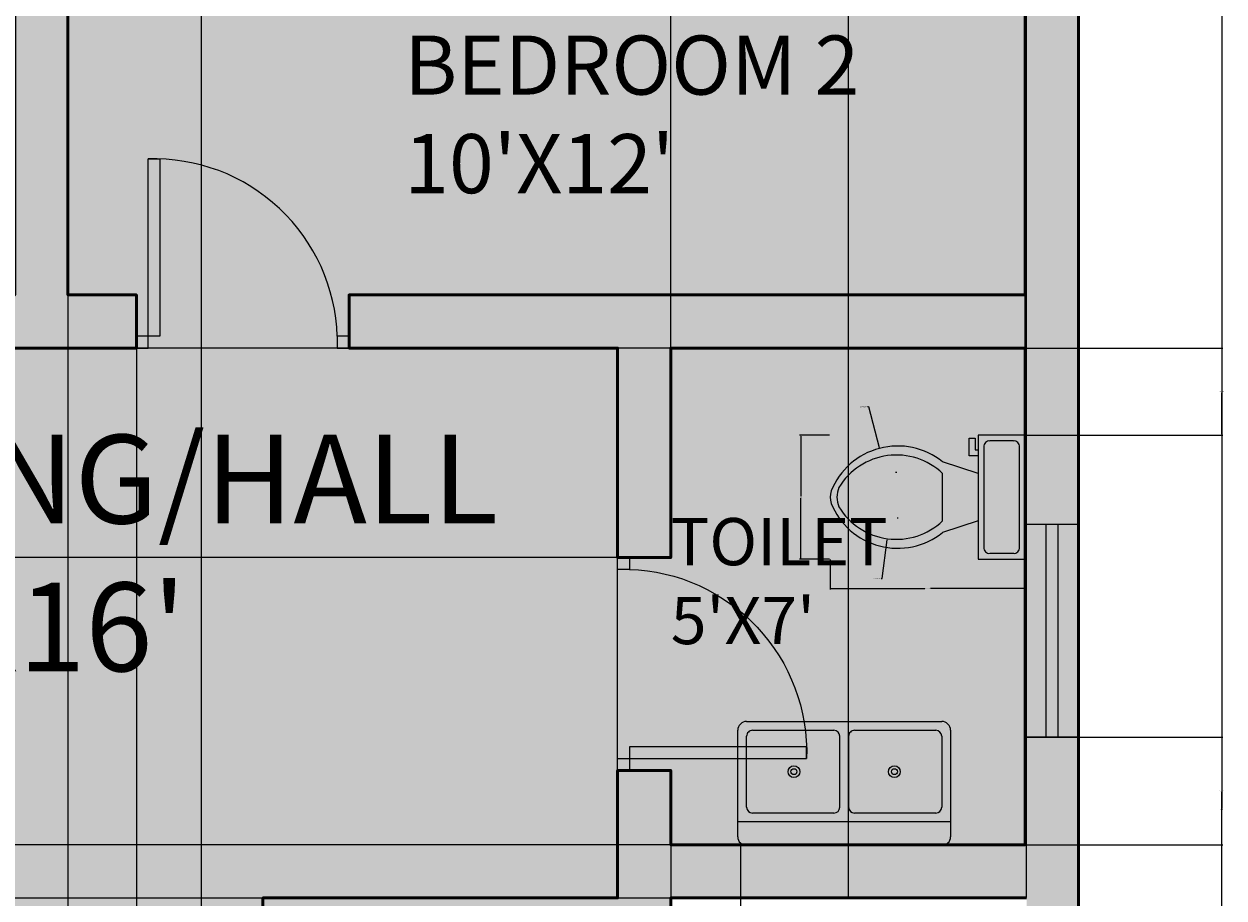
# Model space of a CAD drawing. Units: inches. Extents: x -494 to 1275, y 12 to 1194.
# Tile 3 of 8: x 293 to 496, y 596 to 743. Entities that reach past the tile are written whole.
import ezdxf

# ---------------------------------------------------------------- set-up
doc = ezdxf.new("R2010")
doc.units = ezdxf.units.IN
doc.header["$MEASUREMENT"] = 0
for name, color, linetype, lineweight in [('A-ANNO-DIMS', 2, 'Continuous', 18), ('A-AREA-IDEN', 7, 'Continuous', 25), ('A-DOOR', 3, 'Continuous', 25), ('A-DOOR-PATT', 7, 'Continuous', 13), ('A-FLOR-FIXT', 8, 'Continuous', 18), ('A-GLAZ', 4, 'Continuous', 18), ('A-GLAZ-FRAM-PATT', 7, 'Continuous', 13), ('A-GLAZ-GLAS-PATT', 4, 'Continuous', 13), ('A-WALL', 7, 'Continuous', 50)]:
    doc.layers.add(name, color=color, linetype=linetype, lineweight=lineweight)
doc.layers.add('A-FLOR-PATT', color=51, linetype='Continuous', lineweight=13, true_color=0xf8f6b0)
doc.layers.add('A-WALL-PATT', color=251, linetype='Continuous', lineweight=13, true_color=0x636466)
doc.styles.get("Standard").update_dxf_attribs({"font": 'arial.ttf'})
doc.dimstyles.get("Standard").update_dxf_attribs({"dimtxt": 0.18, "dimasz": 0.18, "dimexe": 0.18, "dimexo": 0.0625, "dimgap": 0.09, "dimtad": 0, "dimtih": 1, "dimtoh": 1, "dimdec": 4, "dimzin": 0, "dimdsep": 46, "dimlunit": 4, "dimtxsty": 'Standard', "dimcen": 0.09, "dimadec": 0, "dimazin": 0, "dimtfac": 1, "dimtdec": 4, "dimtofl": 0, "dimtmove": 0, "dimatfit": 3, "dimfxl": 1, "dimtolj": 1, "dimtzin": 0, "dimarcsym": 0})

# ---------------------------------------------------------------- blocks, each defined once
blk = doc.blocks.new('Toilet - top')
for p, q in [((9.5, -6), (9.5, -2)), ((-8, -8.5), (-8, -8)), ((-7, -8), (-7, -9.5)), ((-4, -8), (-6, -14)), ((4, -8), (6, -14)), ((-10, -8.5), (-8, -8.5)), ((-10, -9.5), (-10, -8.5)), ((-7, -9.5), (-10, -9.5)), ((4, -14), (-4, -14))]:
    blk.add_line(p, q)
blk.add_lwpolyline([(10.5, -8), (10.5, 0), (-10.5, 0), (-10.5, -8)], close=True)
for points in [[(-9.5, -2), (-9.5, -6)], [(8.5, -1), (-8.5, -1)], [(-8.5, -7), (8.5, -7)]]:
    blk.add_lwpolyline(points)
for centre, radius, start, end in [((-8.62, -1.88), 0.884, 81.8699, 188.1301), ((8.62, -1.88), 0.884, 351.8699, 98.1301), ((-8.62, -6.12), 0.884, 171.8699, 278.1301), ((8.62, -6.12), 0.884, 261.8699, 8.1301), ((3.52, -21.58), 12.17, 141.4691, 247.9714), ((4.2, -21.82), 11.33, 136.3677, 238.9468), ((-3.52, -21.58), 12.17, 292.0284, 38.5307), ((-4.2, -21.82), 11.33, 301.053, 43.6321), ((0, -27.88), 4, 245.7318, 294.2682), ((0, -29), 4, 254.8605, 285.1395)]:
    blk.add_arc(centre, radius, start, end)
blk = doc.blocks.new('Sink-double - 36 in top')
for p, q in [((-18, -4), (18, -4)), ((-0.75, -18.5), (-0.75, -6.5)), ((0.75, -6.5), (0.75, -18.5))]:
    blk.add_line(p, q)
for points in [[(-16.5, 0), (16.5, 0)], [(-18, -19.5), (-18, -1.5)], [(18, -1.5), (18, -19.5)], [(-15.5, -5.5), (-1.75, -5.5)], [(1.75, -5.5), (15.5, -5.5)], [(-16.5, -18.5), (-16.5, -6.5)], [(16.5, -6.5), (16.5, -18.5)], [(-1.75, -19.5), (-15.5, -19.5)], [(15.5, -19.5), (1.75, -19.5)], [(16.5, -21), (-16.5, -21)]]:
    blk.add_lwpolyline(points)
for centre, radius in [((-8.5, -12.5), 1), ((-8.5, -12.5), 0.5), ((8.5, -12.5), 1), ((8.5, -12.5), 0.5)]:
    blk.add_circle(centre, radius)
for centre, radius, start, end in [((-16.5, -1.5), 1.5, 90, 180), ((16.5, -1.5), 1.5, 0, 90), ((-15.5, -6.5), 1, 90, 180), ((-1.75, -6.5), 1, 0, 90), ((1.75, -6.5), 1, 90, 180), ((15.5, -6.5), 1, 0, 90), ((-16.5, -19.5), 1.5, 180, 270), ((-15.5, -18.5), 1, 180, 270), ((-1.75, -18.5), 1, 270, 0), ((1.75, -18.5), 1, 180, 270), ((15.5, -18.5), 1, 270, 0), ((16.5, -19.5), 1.5, 270, 0)]:
    blk.add_arc(centre, radius, start, end)
blk = doc.blocks.new('WINDOW-36IN')
for p, q in [((3.5, 36), (3.5, 0)), ((5.5, 36), (5.5, 0))]:
    blk.add_line(p, q)
blk.add_lwpolyline([(0, 36), (9, 36), (9, 0), (0, 0)], close=True)
blk = doc.blocks.new('DOOR-SINGLE-36IN')
blk.add_lwpolyline([(34, 2, 0.414214), (2, 32), (4, 32), (4, 2), (2, 2), (2, 32)], format="xyb")
for points in [[(0, 0), (2, 0), (2, 2), (0, 2)], [(34, 0), (36, 0), (36, 2), (34, 2)]]:
    blk.add_lwpolyline(points, close=True)
blk = doc.blocks.new('*D40')
at = {"layer": 'A-ANNO-DIMS', "color": 0, "lineweight": -2, "transparency": 16777216}
for p, q in [((429.69, 652.77), (429.69, 647.69)), ((462.73, 652.77), (462.73, 647.69)), ((429.87, 647.87), (445.74, 647.87)), ((462.55, 647.87), (446.68, 647.87))]:
    blk.add_line(p, q, dxfattribs=at)
at = {"layer": 'A-ANNO-DIMS', "color": 0, "transparency": 16777216}
for points in [[(429.87, 647.9), (429.87, 647.84), (429.69, 647.87)], [(462.55, 647.9), (462.55, 647.84), (462.73, 647.87)]]:
    blk.add_solid(points, dxfattribs=at)
at = {"layer": 'Defpoints', "color": 0, "transparency": 16777216}
for p in [(429.69, 652.83), (462.73, 652.83), (462.73, 647.87)]:
    blk.add_point(p, dxfattribs=at)
at = {"layer": 'A-ANNO-DIMS', "color": 0, "transparency": 16777216, "insert": (446.21, 647.87), "char_height": 0.18, "attachment_point": 5}
blk.add_mtext('\\A1;WC 33', dxfattribs=at)
blk = doc.blocks.new('*D41')
at = {"layer": 'A-ANNO-DIMS', "color": 0, "lineweight": -2, "transparency": 16777216}
for p, q in [((429.62, 673.83), (424.55, 673.83)), ((424.73, 673.65), (424.73, 663.51)), ((424.73, 653.01), (424.73, 663.15)), ((429.62, 652.83), (424.55, 652.83))]:
    blk.add_line(p, q, dxfattribs=at)
at = {"layer": 'A-ANNO-DIMS', "color": 0, "transparency": 16777216}
for points in [[(424.7, 673.65), (424.76, 673.65), (424.73, 673.83)], [(424.7, 653.01), (424.76, 653.01), (424.73, 652.83)]]:
    blk.add_solid(points, dxfattribs=at)
at = {"layer": 'Defpoints', "color": 0, "transparency": 16777216}
for p in [(429.69, 673.83), (424.73, 652.83), (429.69, 652.83)]:
    blk.add_point(p, dxfattribs=at)
at = {"layer": 'A-ANNO-DIMS', "color": 0, "transparency": 16777216, "insert": (424.73, 663.33), "char_height": 0.18, "attachment_point": 5}
blk.add_mtext('\\A1;21', dxfattribs=at)
blk = doc.blocks.new('*D43')
at = {"layer": 'A-ANNO-DIMS', "color": 0, "lineweight": -2, "transparency": 16777216}
for p, q in [((471.79, 850.53), (496.16, 850.53)), ((495.98, 850.35), (495.98, 610.72)), ((495.98, 370.71), (495.98, 610.35)), ((471.79, 370.53), (496.16, 370.53))]:
    blk.add_line(p, q, dxfattribs=at)
at = {"layer": 'A-ANNO-DIMS', "color": 0, "transparency": 16777216}
for points in [[(495.95, 850.35), (496.01, 850.35), (495.98, 850.53)], [(495.95, 370.71), (496.01, 370.71), (495.98, 370.53)]]:
    blk.add_solid(points, dxfattribs=at)
at = {"layer": 'Defpoints', "color": 0, "transparency": 16777216}
for p in [(471.73, 850.53), (495.98, 850.53), (471.73, 370.53)]:
    blk.add_point(p, dxfattribs=at)
at = {"layer": 'A-ANNO-DIMS', "color": 0, "transparency": 16777216, "insert": (495.98, 610.53), "char_height": 0.18, "attachment_point": 5}
blk.add_mtext('\\A1;480', dxfattribs=at)
blk = doc.blocks.new('*D53')
at = {"layer": 'A-ANNO-DIMS', "color": 0, "lineweight": -2, "transparency": 16777216}
for p, q in [((300.73, 697.47), (300.73, 346.1)), ((312.31, 688.47), (312.31, 346.1)), ((300.91, 346.28), (306.07, 346.28)), ((312.13, 346.28), (306.98, 346.28))]:
    blk.add_line(p, q, dxfattribs=at)
at = {"layer": 'A-ANNO-DIMS', "color": 0, "transparency": 16777216}
for points in [[(300.91, 346.31), (300.91, 346.25), (300.73, 346.28)], [(312.13, 346.31), (312.13, 346.25), (312.31, 346.28)]]:
    blk.add_solid(points, dxfattribs=at)
at = {"layer": 'Defpoints', "color": 0, "transparency": 16777216}
for p in [(300.73, 697.53), (312.31, 688.53), (312.31, 346.28)]:
    blk.add_point(p, dxfattribs=at)
at = {"layer": 'A-ANNO-DIMS', "color": 0, "transparency": 16777216, "insert": (306.52, 346.28), "char_height": 0.18, "attachment_point": 5}
blk.add_mtext('\\A1;11.577', dxfattribs=at)
blk = doc.blocks.new('*D55')
at = {"layer": 'A-ANNO-DIMS', "color": 0, "lineweight": -2, "transparency": 16777216}
for p, q in [((402.67, 688.53), (87.3, 688.53)), ((87.48, 688.35), (87.48, 646.72)), ((87.48, 604.71), (87.48, 646.35)), ((402.67, 604.53), (87.3, 604.53))]:
    blk.add_line(p, q, dxfattribs=at)
at = {"layer": 'A-ANNO-DIMS', "color": 0, "transparency": 16777216}
for points in [[(87.45, 688.35), (87.51, 688.35), (87.48, 688.53)], [(87.45, 604.71), (87.51, 604.71), (87.48, 604.53)]]:
    blk.add_solid(points, dxfattribs=at)
at = {"layer": 'Defpoints', "color": 0, "transparency": 16777216}
for p in [(87.48, 688.53), (402.73, 688.53), (402.73, 604.53)]:
    blk.add_point(p, dxfattribs=at)
at = {"layer": 'A-ANNO-DIMS', "color": 0, "transparency": 16777216, "insert": (87.48, 646.53), "char_height": 0.18, "attachment_point": 5}
blk.add_mtext('\\A1;84', dxfattribs=at)
blk = doc.blocks.new('*D56')
at = {"layer": 'A-ANNO-DIMS', "color": 0, "lineweight": -2, "transparency": 16777216}
for p, q in [((402.73, 688.6), (402.73, 874.96)), ((402.91, 874.78), (432.51, 874.78)), ((462.55, 874.78), (432.95, 874.78)), ((462.73, 688.6), (462.73, 874.96))]:
    blk.add_line(p, q, dxfattribs=at)
at = {"layer": 'A-ANNO-DIMS', "color": 0, "transparency": 16777216}
for points in [[(402.91, 874.81), (402.91, 874.75), (402.73, 874.78)], [(462.55, 874.81), (462.55, 874.75), (462.73, 874.78)]]:
    blk.add_solid(points, dxfattribs=at)
at = {"layer": 'Defpoints', "color": 0, "transparency": 16777216}
for p in [(462.73, 874.78), (402.73, 688.53), (462.73, 688.53)]:
    blk.add_point(p, dxfattribs=at)
at = {"layer": 'A-ANNO-DIMS', "color": 0, "transparency": 16777216, "insert": (432.73, 874.78), "char_height": 0.18, "attachment_point": 5}
blk.add_mtext('\\A1;60', dxfattribs=at)
blk = doc.blocks.new('*D58')
at = {"layer": 'A-ANNO-DIMS', "color": 0, "lineweight": -2, "transparency": 16777216}
for p, q in [((462.79, 622.76), (496.16, 622.76)), ((495.98, 622.58), (495.98, 613.83)), ((495.98, 604.71), (495.98, 613.47)), ((462.79, 604.53), (496.16, 604.53))]:
    blk.add_line(p, q, dxfattribs=at)
at = {"layer": 'A-ANNO-DIMS', "color": 0, "transparency": 16777216}
for points in [[(495.95, 622.58), (496.01, 622.58), (495.98, 622.76)], [(495.95, 604.71), (496.01, 604.71), (495.98, 604.53)]]:
    blk.add_solid(points, dxfattribs=at)
at = {"layer": 'Defpoints', "color": 0, "transparency": 16777216}
for p in [(462.73, 622.76), (495.98, 622.76), (462.73, 604.53)]:
    blk.add_point(p, dxfattribs=at)
at = {"layer": 'A-ANNO-DIMS', "color": 0, "transparency": 16777216, "insert": (495.98, 613.65), "char_height": 0.18, "attachment_point": 5}
blk.add_mtext('\\A1;18.227', dxfattribs=at)
blk = doc.blocks.new('*D61')
at = {"layer": 'A-ANNO-DIMS', "color": 0, "lineweight": -2, "transparency": 16777216}
for p, q in [((393.67, 688.53), (87.3, 688.53)), ((87.48, 688.35), (87.48, 671.01)), ((87.48, 653.3), (87.48, 670.64)), ((393.67, 653.12), (87.3, 653.12))]:
    blk.add_line(p, q, dxfattribs=at)
at = {"layer": 'A-ANNO-DIMS', "color": 0, "transparency": 16777216}
for points in [[(87.45, 688.35), (87.51, 688.35), (87.48, 688.53)], [(87.45, 653.3), (87.51, 653.3), (87.48, 653.12)]]:
    blk.add_solid(points, dxfattribs=at)
at = {"layer": 'Defpoints', "color": 0, "transparency": 16777216}
for p in [(393.73, 688.53), (87.48, 653.12), (393.73, 653.12)]:
    blk.add_point(p, dxfattribs=at)
at = {"layer": 'A-ANNO-DIMS', "color": 0, "transparency": 16777216, "insert": (87.48, 670.83), "char_height": 0.18, "attachment_point": 5}
blk.add_mtext('\\A1;35.416', dxfattribs=at)
blk = doc.blocks.new('*D63')
at = {"layer": 'A-ANNO-DIMS', "color": 0, "lineweight": -2, "transparency": 16777216}
for p, q in [((402.67, 595.53), (87.3, 595.53)), ((87.48, 595.35), (87.48, 487.72)), ((87.48, 379.71), (87.48, 487.35)), ((342.67, 379.53), (87.3, 379.53))]:
    blk.add_line(p, q, dxfattribs=at)
at = {"layer": 'A-ANNO-DIMS', "color": 0, "transparency": 16777216}
for points in [[(87.45, 595.35), (87.51, 595.35), (87.48, 595.53)], [(87.45, 379.71), (87.51, 379.71), (87.48, 379.53)]]:
    blk.add_solid(points, dxfattribs=at)
at = {"layer": 'Defpoints', "color": 0, "transparency": 16777216}
for p in [(402.73, 595.53), (87.48, 379.53), (342.73, 379.53)]:
    blk.add_point(p, dxfattribs=at)
at = {"layer": 'A-ANNO-DIMS', "color": 0, "transparency": 16777216, "insert": (87.48, 487.53), "char_height": 0.18, "attachment_point": 5}
blk.add_mtext('\\A1;216', dxfattribs=at)
blk = doc.blocks.new('*D64')
at = {"layer": 'A-ANNO-DIMS', "color": 0, "lineweight": -2, "transparency": 16777216}
for p, q in [((432.84, 595.6), (432.84, 874.96)), ((433.02, 874.78), (447.43, 874.78)), ((462.76, 874.78), (448.35, 874.78)), ((462.94, 595.6), (462.94, 874.96))]:
    blk.add_line(p, q, dxfattribs=at)
at = {"layer": 'A-ANNO-DIMS', "color": 0, "transparency": 16777216}
for points in [[(433.02, 874.81), (433.02, 874.75), (432.84, 874.78)], [(462.76, 874.81), (462.76, 874.75), (462.94, 874.78)]]:
    blk.add_solid(points, dxfattribs=at)
at = {"layer": 'Defpoints', "color": 0, "transparency": 16777216}
for p in [(462.94, 874.78), (432.84, 595.53), (462.94, 595.53)]:
    blk.add_point(p, dxfattribs=at)
at = {"layer": 'A-ANNO-DIMS', "color": 0, "transparency": 16777216, "insert": (447.89, 874.78), "char_height": 0.18, "attachment_point": 5}
blk.add_mtext('\\A1;30.104', dxfattribs=at)
blk = doc.blocks.new('*D69')
at = {"layer": 'A-ANNO-DIMS', "color": 0, "lineweight": -2, "transparency": 16777216}
for p, q in [((402.73, 604.47), (402.73, 346.1)), ((414.52, 604.78), (414.52, 346.1)), ((402.91, 346.28), (408.19, 346.28)), ((414.34, 346.28), (409.07, 346.28))]:
    blk.add_line(p, q, dxfattribs=at)
at = {"layer": 'A-ANNO-DIMS', "color": 0, "transparency": 16777216}
for points in [[(402.91, 346.31), (402.91, 346.25), (402.73, 346.28)], [(414.34, 346.31), (414.34, 346.25), (414.52, 346.28)]]:
    blk.add_solid(points, dxfattribs=at)
at = {"layer": 'Defpoints', "color": 0, "transparency": 16777216}
for p in [(402.73, 604.53), (414.52, 604.84), (414.52, 346.28)]:
    blk.add_point(p, dxfattribs=at)
at = {"layer": 'A-ANNO-DIMS', "color": 0, "transparency": 16777216, "insert": (408.63, 346.28), "char_height": 0.18, "attachment_point": 5}
blk.add_mtext('\\A1;11.791', dxfattribs=at)
blk = doc.blocks.new('*D70')
at = {"layer": 'A-ANNO-DIMS', "color": 0, "lineweight": -2, "transparency": 16777216}
for p, q in [((462.79, 688.53), (496.16, 688.53)), ((495.98, 688.35), (495.98, 681.36)), ((495.98, 674.01), (495.98, 681)), ((462.79, 673.83), (496.16, 673.83))]:
    blk.add_line(p, q, dxfattribs=at)
at = {"layer": 'A-ANNO-DIMS', "color": 0, "transparency": 16777216}
for points in [[(495.95, 688.35), (496.01, 688.35), (495.98, 688.53)], [(495.95, 674.01), (496.01, 674.01), (495.98, 673.83)]]:
    blk.add_solid(points, dxfattribs=at)
at = {"layer": 'Defpoints', "color": 0, "transparency": 16777216}
for p in [(462.73, 688.53), (462.73, 673.83), (495.98, 673.83)]:
    blk.add_point(p, dxfattribs=at)
at = {"layer": 'A-ANNO-DIMS', "color": 0, "transparency": 16777216, "insert": (495.98, 681.18), "char_height": 0.18, "attachment_point": 5}
blk.add_mtext('\\A1;14.706', dxfattribs=at)
blk = doc.blocks.new('*D83')
at = {"layer": 'A-ANNO-DIMS', "color": 0, "lineweight": -2, "transparency": 16777216}
for p, q in [((300.73, 820.48), (300.73, 346.1)), ((323.29, 820.48), (323.29, 346.1)), ((300.91, 346.28), (311.55, 346.28)), ((323.11, 346.28), (312.48, 346.28))]:
    blk.add_line(p, q, dxfattribs=at)
at = {"layer": 'A-ANNO-DIMS', "color": 0, "transparency": 16777216}
for points in [[(300.91, 346.31), (300.91, 346.25), (300.73, 346.28)], [(323.11, 346.31), (323.11, 346.25), (323.29, 346.28)]]:
    blk.add_solid(points, dxfattribs=at)
at = {"layer": 'Defpoints', "color": 0, "transparency": 16777216}
for p in [(300.73, 820.54), (323.29, 820.54), (323.29, 346.28)]:
    blk.add_point(p, dxfattribs=at)
at = {"layer": 'A-ANNO-DIMS', "color": 0, "transparency": 16777216, "insert": (312.01, 346.28), "char_height": 0.18, "attachment_point": 5}
blk.add_mtext('\\A1;22.557', dxfattribs=at)
blk = doc.blocks.new('*D98')
at = {"layer": 'A-ANNO-DIMS', "color": 0, "lineweight": -2, "transparency": 16777216}
for p, q in [((436.02, 678.64), (436.2, 678.64)), ((436.2, 678.64), (438.01, 671.75)), ((441.06, 659.81), (441.24, 659.81)), ((441.15, 659.72), (441.15, 659.9))]:
    blk.add_line(p, q, dxfattribs=at)
at = {"layer": 'A-ANNO-DIMS', "color": 0, "transparency": 16777216}
blk.add_solid([(438.04, 671.76), (437.99, 671.75), (438.06, 671.58)], dxfattribs=at)
at = {"layer": 'Defpoints', "color": 0, "transparency": 16777216}
for p in [(438.06, 671.58), (441.15, 659.81)]:
    blk.add_point(p, dxfattribs=at)
at = {"layer": 'A-ANNO-DIMS', "color": 0, "transparency": 16777216, "insert": (435.35, 678.64), "char_height": 0.18, "attachment_point": 5}
blk.add_mtext('\\A1;2X R12.17', dxfattribs=at)
blk = doc.blocks.new('*D99')
at = {"layer": 'A-ANNO-DIMS', "color": 0, "lineweight": -2, "transparency": 16777216}
for p, q in [((440.82, 667.53), (441, 667.53)), ((440.91, 667.44), (440.91, 667.62)), ((438.5, 649.56), (439.38, 656.12)), ((438.32, 649.56), (438.5, 649.56))]:
    blk.add_line(p, q, dxfattribs=at)
at = {"layer": 'A-ANNO-DIMS', "color": 0, "transparency": 16777216}
blk.add_solid([(439.35, 656.13), (439.41, 656.12), (439.4, 656.3)], dxfattribs=at)
at = {"layer": 'Defpoints', "color": 0, "transparency": 16777216}
for p in [(440.91, 667.53), (439.4, 656.3)]:
    blk.add_point(p, dxfattribs=at)
at = {"layer": 'A-ANNO-DIMS', "color": 0, "transparency": 16777216, "insert": (437.64, 649.56), "char_height": 0.18, "attachment_point": 5}
blk.add_mtext('\\A1;2X R11.33', dxfattribs=at)

msp = doc.modelspace()

# ---------------------------------------------------------------- hatches: boundary and pattern name
at = {"layer": 'A-DOOR-PATT'}
h = msp.add_hatch(color=256, dxfattribs=at)
h.dxf.hatch_style = 1
h.paths.add_polyline_path([(316.3096, 720.5349), (314.3096, 720.5349), (314.3096, 690.5349), (316.3096, 690.5349)])
h.paths.add_polyline_path([(314.3096, 690.5349), (312.3096, 690.5349), (312.3096, 688.5349), (314.3096, 688.5349)])
h.paths.add_polyline_path([(348.3096, 690.5349), (346.3096, 690.5349), (346.3096, 688.5349), (348.3096, 688.5349)])
h = msp.add_hatch(color=256, dxfattribs=at)
h.dxf.hatch_style = 1
h.paths.add_polyline_path([(425.7322, 619.1185), (425.7322, 621.1185), (395.7322, 621.1185), (395.7322, 619.1185)])
h.paths.add_polyline_path([(393.7322, 617.1185), (395.7322, 617.1185), (395.7322, 619.1185), (393.7322, 619.1185)])
h.paths.add_polyline_path([(393.7322, 653.1185), (393.7322, 651.1185), (395.7322, 651.1185), (395.7322, 653.1185)])
at = {"layer": 'A-FLOR-PATT'}
h = msp.add_hatch(color=256, dxfattribs=at)
h.dxf.hatch_style = 1
h.paths.add_polyline_path([(333.7322, 595.5349), (393.7322, 595.5349), (393.7322, 617.1185), (393.7322, 653.1185), (393.7322, 688.5349), (348.3096, 688.5349), (348.3096, 697.5349), (462.7322, 697.5349), (462.7322, 841.5349), (300.7322, 841.5349), (300.7322, 820.5433), (323.2889, 820.5433), (323.2889, 769.5349), (300.7322, 769.5349), (300.7322, 697.5349), (312.3096, 697.5349), (312.3096, 688.5349), (276.4565, 688.5349), (276.4565, 697.5349), (291.7322, 697.5349), (291.7322, 771.5415), (264.338, 771.5415), (264.338, 820.5433), (291.7322, 820.5433), (291.7322, 841.5349), (120.7322, 841.5349), (120.7322, 697.5349), (240.4565, 697.5349), (240.4565, 688.5349), (120.7322, 688.5349), (120.7322, 451.5349), (241.3385, 451.5349), (241.3385, 442.5349), (277.3385, 442.5349), (277.3385, 451.5349), (333.7322, 451.5349), (333.7322, 473.4986), (333.7322, 509.4986)])
h.paths.add_polyline_path([(372.4977, 745.1275), (372.4977, 805.1275), (452.4977, 805.1275), (452.4977, 745.1275)], flags=16)
h.paths.add_polyline_path([(208.4976, 745.1275), (128.4976, 745.1275), (128.4976, 805.1275), (208.4976, 805.1275)], flags=16)
h.paths.add_polyline_path([(422.8977, 745.1275), (422.8977, 760.3275), (438.0977, 760.3275), (438.0977, 797.1275), (451.2977, 797.1275), (451.2977, 776.3275), (438.0977, 776.3275), (438.0977, 773.9275), (451.2977, 773.9275), (451.2977, 753.1275), (436.0977, 753.1275), (436.0977, 758.3275)], flags=16)
h.paths.add_polyline_path([(142.8976, 789.9275), (142.8976, 753.1275), (129.6976, 753.1275), (129.6976, 773.9275), (142.8976, 773.9275), (142.8976, 776.3275), (129.6976, 776.3275), (129.6976, 797.1275), (144.8976, 797.1275), (144.8976, 791.9275), (158.0976, 805.1275), (158.0976, 789.9275)], flags=0)
h = msp.add_hatch(color=256, dxfattribs=at)
h.dxf.hatch_style = 1
h.paths.add_polyline_path([(462.7322, 688.5349), (402.7322, 688.5349), (402.7322, 653.1185), (393.7322, 653.1185), (393.7322, 617.1185), (402.7322, 617.1185), (402.7322, 604.5349), (462.7322, 604.5349)])
at = {"layer": 'A-GLAZ-FRAM-PATT'}
h = msp.add_hatch(color=256, dxfattribs=at)
h.dxf.hatch_style = 1
h.paths.add_polyline_path([(466.2322, 658.762), (462.7322, 658.762), (462.7322, 622.762), (466.2322, 622.762)])
h.paths.add_polyline_path([(471.7322, 658.762), (468.2322, 658.762), (468.2322, 622.762), (471.7322, 622.762)])
at = {"layer": 'A-GLAZ-GLAS-PATT'}
h = msp.add_hatch(color=256, dxfattribs=at)
h.dxf.hatch_style = 1
h.paths.add_polyline_path([(468.2322, 658.762), (466.2322, 658.762), (466.2322, 622.762), (468.2322, 622.762)])
at = {"layer": 'A-WALL-PATT'}
h = msp.add_hatch(color=256, dxfattribs=at)
h.dxf.hatch_style = 1
h.paths.add_polyline_path([(120.7322, 841.5349), (291.7322, 841.5349), (291.7322, 697.5349), (276.4565, 697.5349), (276.4565, 688.5349), (312.3096, 688.5349), (312.3096, 697.5349), (300.7322, 697.5349), (300.7322, 841.5349), (462.7322, 841.5349), (462.7322, 697.5349), (348.3096, 697.5349), (348.3096, 688.5349), (393.7322, 688.5349), (393.7322, 653.1185), (402.7322, 653.1185), (402.7322, 688.5349), (462.7322, 688.5349), (462.7322, 604.5349), (402.7322, 604.5349), (402.7322, 617.1185), (393.7322, 617.1185), (393.7322, 595.5349), (333.7322, 595.5349), (333.7322, 509.4986), (342.7322, 509.4986), (342.7322, 586.5349), (393.7322, 586.5349), (402.7322, 586.5349), (402.7322, 595.5349), (462.9409, 595.5349), (462.7406, 379.5349), (342.7322, 379.5349), (342.7322, 442.5349), (342.7322, 473.4986), (333.7322, 473.4986), (333.7322, 451.5349), (277.3385, 451.5349), (277.3385, 442.5349), (333.7322, 442.5349), (333.7322, 370.5349), (471.7322, 370.5349), (471.7322, 850.5349), (111.7322, 850.5349), (111.7322, 442.5349), (241.3385, 442.5349), (241.3385, 451.5349), (120.7322, 451.5349), (120.7322, 688.5349), (240.4565, 688.5349), (240.4565, 697.5349), (120.7322, 697.5349)])

# ---------------------------------------------------------------- linework, layer by layer
at = {"layer": 'A-DOOR'}
msp.add_line((393.7322, 617.1185), (393.7322, 653.1185), dxfattribs=at)
at = {"layer": 'A-WALL'}
for points in [[(333.7322, 442.5349), (333.7322, 370.5349), (471.7322, 370.5349), (471.7322, 850.5349), (111.7322, 850.5349), (111.7322, 442.5349), (241.3385, 442.5349), (241.3385, 451.5349), (120.7322, 451.5349), (120.7322, 688.5349), (240.4565, 688.5349), (240.4565, 697.5349), (120.7322, 697.5349), (120.7322, 841.5349), (291.7322, 841.5349), (291.7322, 697.5349), (276.4565, 697.5349), (276.4565, 688.5349), (312.3096, 688.5349), (312.3096, 697.5349), (300.7322, 697.5349), (300.7322, 841.5349)], [(462.9409, 595.5349), (402.7322, 595.5349), (402.7322, 586.5349), (393.7322, 586.5349), (342.7322, 586.5349), (342.7322, 509.4986), (333.7322, 509.4986), (333.7322, 595.5349), (393.7322, 595.5349), (393.7322, 617.1185), (402.7322, 617.1185), (402.7322, 604.5349), (462.7322, 604.5349), (462.7322, 688.5349), (402.7322, 688.5349), (402.7322, 653.1185), (393.7322, 653.1185), (393.7322, 688.5349), (348.3096, 688.5349), (348.3096, 697.5349), (462.7322, 697.5349), (462.7322, 841.5349), (300.7322, 841.5349)]]:
    msp.add_lwpolyline(points, dxfattribs=at)

# ---------------------------------------------------------------- block references
at = {"layer": 'A-DOOR'}
msp.add_blockref('DOOR-SINGLE-36IN', (312.3099, 688.535), dxfattribs=at)
at = {"layer": 'A-DOOR', "extrusion": (0, 0, -1), "zscale": -1, "rotation": 90.00000000000017}
msp.add_blockref('DOOR-SINGLE-36IN', (-393.7323, 617.1189), dxfattribs=at)
at = {"layer": 'A-FLOR-FIXT'}
for name, p, rotation in [('Toilet - top', (462.7322, 663.3291), 270), ('Sink-double - 36 in top', (432.0841, 604.3983), 180)]:
    msp.add_blockref(name, p, dxfattribs=dict(at, rotation=rotation))
at = {"layer": 'A-GLAZ'}
msp.add_blockref('WINDOW-36IN', (462.732, 622.762), dxfattribs=at)

# ---------------------------------------------------------------- texts
at = {"layer": 'A-AREA-IDEN', "attachment_point": 1}
for s, width, insert, char_height in [("BEDROOM 2\\P10'X12'", 95.40663, (357.6461, 741.4086), 10), ("LIVING/HALL\\P14'X16'", 130.54611, (252.1968, 673.8839), 15), ("TOILET\\P5'X7'", 47.525183, (402.7322, 659.8042), 8)]:
    msp.add_mtext_dynamic_manual_height_columns(s, width=width, gutter_width=1, heights=[0], dxfattribs=dict(at, insert=insert, char_height=char_height))

# ---------------------------------------------------------------- dimensions: what is measured, and where the dimension line sits
at = {"layer": 'A-ANNO-DIMS'}
for base, p1, p2, override, picture, middle in [((462.7322, 874.7849), (402.7322, 688.5349), (462.7322, 688.5349), {"dimdec": 0, "dimlfac": 1, "dimrnd": 0, "dimzin": 0, "dimdsep": 46, "dimlunit": 2}, '*D56', (432.7322, 874.7849)), ((462.9409, 874.7849), (432.8366, 595.5349), (462.9409, 595.5349), {"dimdec": 3, "dimlfac": 1, "dimrnd": 0, "dimzin": 0, "dimdsep": 46, "dimlunit": 2}, '*D64', (447.8888, 874.7849)), ((323.2889, 346.2849), (300.7322, 820.5433), (323.2889, 820.5433), {"dimdec": 3, "dimlfac": 1, "dimrnd": 0, "dimzin": 0, "dimdsep": 46, "dimlunit": 2}, '*D83', (312.0106, 346.2849)), ((312.3096, 346.2849), (300.7322, 697.5349), (312.3096, 688.5349), {"dimdec": 3, "dimlfac": 1, "dimrnd": 0, "dimzin": 0, "dimdsep": 46, "dimlunit": 2}, '*D53', (306.5209, 346.2849)), ((414.5234, 346.2849), (402.7322, 604.5349), (414.5234, 604.8376), {"dimdec": 3, "dimlfac": 1, "dimrnd": 0, "dimzin": 0, "dimdsep": 46, "dimlunit": 2}, '*D69', (408.6278, 346.2849))]:
    dim = msp.add_linear_dim(base=base, p1=p1, p2=p2, dimstyle='Standard', override=override, dxfattribs=at)
    dim.commit()
    dim.dimension.update_dxf_attribs({"geometry": picture, "text_midpoint": middle})
for base, p1, p2, angle, override, picture, middle in [((495.9822, 850.5349), (471.7322, 370.5349), (471.7322, 850.5349), 90, {"dimdec": 0, "dimlfac": 1, "dimrnd": 0, "dimzin": 0, "dimdsep": 46, "dimlunit": 2}, '*D43', (495.9822, 610.5349)), ((87.4822, 653.1185), (393.7322, 688.5349), (393.7322, 653.1185), 90, {"dimdec": 3, "dimlfac": 1, "dimrnd": 0, "dimzin": 0, "dimdsep": 46, "dimlunit": 2}, '*D61', (87.4822, 670.8267)), ((87.4822, 688.5349), (402.7322, 604.5349), (402.7322, 688.5349), 90, {"dimdec": 0, "dimlfac": 1, "dimrnd": 0, "dimzin": 0, "dimdsep": 46, "dimlunit": 2}, '*D55', (87.4822, 646.5349)), ((495.9822, 673.8291), (462.7322, 688.5349), (462.7322, 673.8291), 90, {"dimdec": 3, "dimlfac": 1, "dimrnd": 0, "dimzin": 0, "dimdsep": 46, "dimlunit": 2}, '*D70', (495.9822, 681.182)), ((424.729, 652.8291), (429.686, 673.8291), (429.686, 652.8291), 270, {"dimdec": 0, "dimlfac": 1, "dimrnd": 0, "dimzin": 0, "dimdsep": 46, "dimlunit": 2}, '*D41', (424.729, 663.3291)), ((495.9822, 622.762), (462.7322, 604.5349), (462.7322, 622.762), 90, {"dimdec": 3, "dimlfac": 1, "dimrnd": 0, "dimzin": 0, "dimdsep": 46, "dimlunit": 2}, '*D58', (495.9822, 613.6484)), ((87.4822, 379.5349), (402.7322, 595.5349), (342.7322, 379.5349), 90, {"dimdec": 0, "dimlfac": 1, "dimrnd": 0, "dimzin": 0, "dimdsep": 46, "dimlunit": 2}, '*D63', (87.4822, 487.5349))]:
    dim = msp.add_linear_dim(base=base, p1=p1, p2=p2, angle=angle, dimstyle='Standard', override=override, dxfattribs=at)
    dim.commit()
    dim.dimension.update_dxf_attribs({"geometry": picture, "text_midpoint": middle})
for center, mpoint, picture, middle in [((441.1517, 659.8095), (438.0599, 671.5792), '*D98', (435.3501, 678.641)), ((440.9148, 667.529), (439.405, 656.3008), '*D99', (437.6443, 649.5639))]:
    dim = msp.add_radius_dim(center=center, mpoint=mpoint, text='2X <>', dimstyle='Standard', override={"dimdec": 2, "dimlfac": 1, "dimrnd": 0, "dimzin": 0, "dimdsep": 46, "dimlunit": 2}, dxfattribs=at)
    dim.commit()
    dim.dimension.update_dxf_attribs({"geometry": picture, "text_midpoint": middle, "dimtype": 164})
dim = msp.add_linear_dim(base=(462.7322, 647.8721), p1=(429.686, 652.8291), p2=(462.7322, 652.8291), text='WC <>', dimstyle='Standard', override={"dimdec": 0, "dimlfac": 1, "dimrnd": 0, "dimzin": 0, "dimdsep": 46, "dimlunit": 2}, dxfattribs=at)
dim.commit()
dim.dimension.update_dxf_attribs({"geometry": '*D40', "text_midpoint": (446.2091, 647.8721)})

doc.saveas('drawing.dxf')
